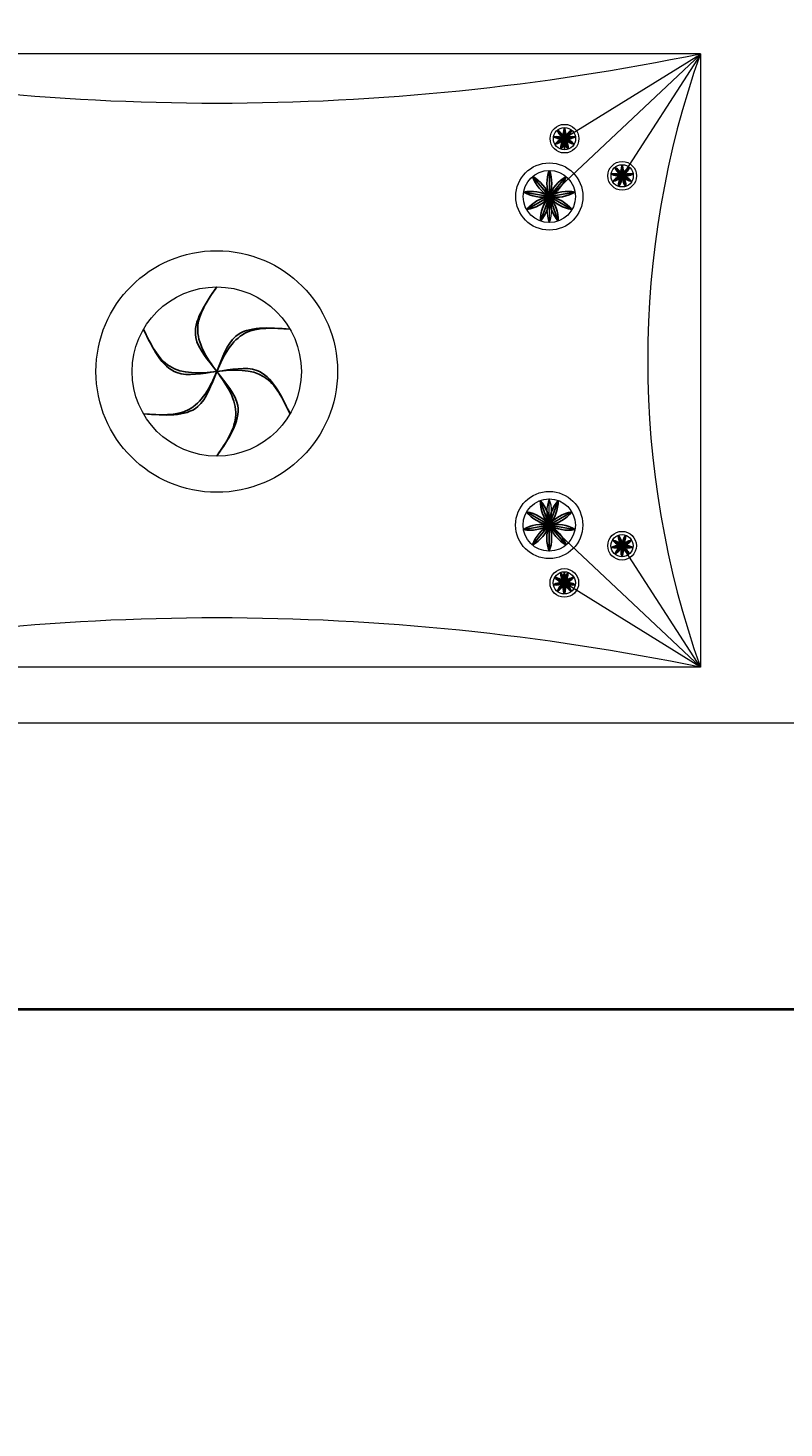
# Model space of a CAD drawing. Units: inches. Extents: x -46 to 1145, y -527 to 760.
# Tile 26 of 57: x 63 to 79, y 222 to 252. Entities that reach past the tile are written whole.
import ezdxf

# ---------------------------------------------------------------- set-up
doc = ezdxf.new("R2010")
doc.units = ezdxf.units.IN
doc.header["$MEASUREMENT"] = 0
for name, color, linetype, lineweight in [('A-ANNO-DIMS', 2, 'Continuous', 18), ('A-FURN', 2, 'Continuous', 13), ('WALLS', 4, 'Continuous', 40)]:
    doc.layers.add(name, color=color, linetype=linetype, lineweight=lineweight)
doc.layers.add('FURNTIURE', color=2, linetype='Continuous')
doc.layers.add('LT', color=9, linetype='Continuous')
doc.styles.get("Standard").update_dxf_attribs({"font": 'arial.ttf'})
doc.dimstyles.get("Standard").update_dxf_attribs({"dimtxt": 0.18, "dimasz": 0.18, "dimexe": 0.18, "dimexo": 0.0625, "dimgap": 0.09, "dimtad": 0, "dimtih": 1, "dimtoh": 1, "dimdec": 0, "dimzin": 0, "dimdsep": 46, "dimlunit": 3, "dimtxsty": 'Standard', "dimcen": 0.09, "dimadec": 0, "dimazin": 0, "dimtfac": 1, "dimtdec": 0, "dimtofl": 0, "dimtmove": 0, "dimatfit": 3, "dimfxl": 1, "dimtolj": 1, "dimtzin": 0, "dimarcsym": 0})

# ---------------------------------------------------------------- blocks, each defined once
blk = doc.blocks.new('*U64')
at = {"layer": 'LT'}
blk.add_line((0, 0.281), (0, -0.281), dxfattribs=at)
for centre, start, end in [((0.734, 0), 159.0676, 200.9324), ((-0.734, 0), 339.0676, 20.9324)]:
    blk.add_arc(centre, 0.786, start, end, dxfattribs=at)
blk = doc.blocks.new('*U65')
at = {"layer": 'LT', "transparency": 16777216}
blk.add_blockref('*U64', (609.936, 444.026), dxfattribs=at)
for p, rotation in [((609.756, 443.96), 40.00000000000002), ((610.117, 443.96), 320), ((609.659, 443.794), 80.00000000000001), ((609.693, 443.605), 120), ((609.84, 443.481), 160), ((610.032, 443.481), 200), ((610.179, 443.605), 240), ((610.213, 443.794), 280)]:
    blk.add_blockref('*U64', p, dxfattribs=dict(at, rotation=rotation))
blk = doc.blocks.new('*U66')
at = {"layer": 'LT'}
blk.add_line((0, 0.12), (0, -0.12), dxfattribs=at)
for centre, start, end in [((0.313, 0), 159.0676, 200.9324), ((-0.313, 0), 339.0676, 20.9324)]:
    blk.add_arc(centre, 0.335, start, end, dxfattribs=at)
blk = doc.blocks.new('*U67')
at = {"layer": 'LT', "transparency": 16777216}
for p, rotation in [((259.495, 188.896), 80.00000000000001), ((259.509, 188.816), 120), ((259.536, 188.967), 40), ((259.572, 188.763), 160), ((259.654, 188.763), 200), ((259.69, 188.967), 320), ((259.716, 188.816), 240), ((259.731, 188.896), 280)]:
    blk.add_blockref('*U66', p, dxfattribs=dict(at, rotation=rotation))
blk.add_blockref('*U66', (259.613, 188.995), dxfattribs=at)
blk = doc.blocks.new('*U68')
at = {"layer": 'LT'}
blk.add_line((0, 0.12), (0, -0.12), dxfattribs=at)
for centre, start, end in [((0.313, 0), 159.0676, 200.9324), ((-0.313, 0), 339.0676, 20.9324)]:
    blk.add_arc(centre, 0.335, start, end, dxfattribs=at)
blk = doc.blocks.new('*U69')
at = {"layer": 'LT', "transparency": 16777216}
for p, rotation in [((259.495, 188.896), 80.00000000000001), ((259.509, 188.816), 120), ((259.536, 188.967), 40), ((259.572, 188.763), 160), ((259.654, 188.763), 200), ((259.69, 188.967), 320), ((259.716, 188.816), 240), ((259.731, 188.896), 280)]:
    blk.add_blockref('*U68', p, dxfattribs=dict(at, rotation=rotation))
blk.add_blockref('*U68', (259.613, 188.995), dxfattribs=at)
blk = doc.blocks.new('*U50')
at = {"layer": 'LT'}
blk.add_line((0, 0.281), (0, -0.281), dxfattribs=at)
for centre, start, end in [((0.734, 0), 159.0676, 200.9324), ((-0.734, 0), 339.0676, 20.9324)]:
    blk.add_arc(centre, 0.786, start, end, dxfattribs=at)
blk = doc.blocks.new('*U51')
at = {"layer": 'LT', "transparency": 16777216}
blk.add_blockref('*U50', (609.936, 444.026), dxfattribs=at)
for p, rotation in [((609.756, 443.96), 40.00000000000002), ((610.117, 443.96), 320), ((609.659, 443.794), 80.00000000000001), ((609.693, 443.605), 120), ((609.84, 443.481), 160), ((610.032, 443.481), 200), ((610.179, 443.605), 240), ((610.213, 443.794), 280)]:
    blk.add_blockref('*U50', p, dxfattribs=dict(at, rotation=rotation))
blk = doc.blocks.new('*U52')
at = {"layer": 'LT'}
blk.add_line((0, 0.12), (0, -0.12), dxfattribs=at)
for centre, start, end in [((0.313, 0), 159.0676, 200.9324), ((-0.313, 0), 339.0676, 20.9324)]:
    blk.add_arc(centre, 0.335, start, end, dxfattribs=at)
blk = doc.blocks.new('*U53')
at = {"layer": 'LT', "transparency": 16777216}
for p, rotation in [((259.495, 188.896), 80.00000000000001), ((259.509, 188.816), 120), ((259.536, 188.967), 40), ((259.572, 188.763), 160), ((259.654, 188.763), 200), ((259.69, 188.967), 320), ((259.716, 188.816), 240), ((259.731, 188.896), 280)]:
    blk.add_blockref('*U52', p, dxfattribs=dict(at, rotation=rotation))
blk.add_blockref('*U52', (259.613, 188.995), dxfattribs=at)
blk = doc.blocks.new('*U54')
at = {"layer": 'LT'}
blk.add_line((0, 0.12), (0, -0.12), dxfattribs=at)
for centre, start, end in [((0.313, 0), 159.0676, 200.9324), ((-0.313, 0), 339.0676, 20.9324)]:
    blk.add_arc(centre, 0.335, start, end, dxfattribs=at)
blk = doc.blocks.new('*U55')
at = {"layer": 'LT', "transparency": 16777216}
for p, rotation in [((259.495, 188.896), 80.00000000000001), ((259.509, 188.816), 120), ((259.536, 188.967), 40), ((259.572, 188.763), 160), ((259.654, 188.763), 200), ((259.69, 188.967), 320), ((259.716, 188.816), 240), ((259.731, 188.896), 280)]:
    blk.add_blockref('*U54', p, dxfattribs=dict(at, rotation=rotation))
blk.add_blockref('*U54', (259.613, 188.995), dxfattribs=at)
blk = doc.blocks.new('*U56')
at = {"layer": 'FURNTIURE'}
blk.add_open_spline([(0.039, 1.82), (-0.218, 1.447), (-0.661, 0.801), (0.102, -0.025), (0.645, -0.928), (0.238, -1.527), (0.039, -1.82)], degree=3, knots=[0, 0, 0, 0, 1.177175, 2.037162, 3.056205, 4.032246, 4.032246, 4.032246, 4.032246], dxfattribs=at)
blk = doc.blocks.new('*U57')
at = {"layer": 'FURNTIURE', "transparency": 16777216}
blk.add_blockref('*U56', (904.302, 663.383), dxfattribs=at)
for p, rotation in [((904.379, 663.383), 180), ((904.321, 663.416), 300), ((904.36, 663.416), 239.9999999999999), ((904.321, 663.349), 59.99999999999999), ((904.36, 663.349), 119.9999999999999)]:
    blk.add_blockref('*U56', p, dxfattribs=dict(at, rotation=rotation))
blk = doc.blocks.new('BED-QUEEN-FURNISHED')
for p, q in [((0, 80), (60, 80)), ((31.2, 78.8), (52, 78.8)), ((31.2, 65.6), (31.2, 78.8)), ((31.2, 78.8), (52, 78.8)), ((31.2, 65.6), (31.2, 78.8)), ((31.2, 78.8), (34.585, 75.613)), ((31.2, 78.8), (32.884, 76.184)), ((31.2, 78.8), (34.126, 76.984)), ((34.126, 76.984), (34.126, 76.745)), ((34.451, 75.739), (34.451, 75.177)), ((34.449, 68.673), (34.449, 69.235)), ((31.195, 65.614), (34.582, 68.799)), ((31.195, 65.614), (32.882, 68.228)), ((34.123, 67.428), (34.123, 67.667)), ((31.195, 65.614), (34.123, 67.428)), ((31.2, 65.6), (52, 65.6)), ((31.2, 65.6), (52, 65.6))]:
    blk.add_line(p, q)
for centre, radius in [((34.126, 76.984), 0.308), ((34.126, 76.984), 0.239), ((32.884, 76.184), 0.308), ((32.884, 76.184), 0.239), ((34.451, 75.739), 0.723), ((34.451, 75.739), 0.562), ((41.604, 72.437), 2.599), ((41.604, 72.437), 1.82), ((34.449, 68.673), 0.723), ((34.449, 68.673), 0.562), ((32.882, 68.228), 0.308), ((32.882, 68.228), 0.239), ((34.123, 67.428), 0.308), ((34.123, 67.428), 0.239)]:
    blk.add_circle(centre, radius)
for centre, radius, start, end in [((41.6, 129.177), 51.439, 258.3356, 281.6644), ((12.546, 72.2), 19.787, 340.5151, 19.4849), ((34.439, 76.865), 0.335, 159.0676, 200.9324), ((33.814, 76.865), 0.335, 339.0676, 20.9324), ((35.185, 75.458), 0.786, 159.0676, 200.9324), ((33.717, 75.458), 0.786, 339.0676, 20.9324), ((35.183, 68.953), 0.786, 159.028, 200.8928), ((33.715, 68.954), 0.786, 339.028, 20.8928), ((34.435, 67.547), 0.335, 159.028, 200.8928), ((33.81, 67.548), 0.335, 339.028, 20.8928), ((41.6, 15.223), 51.439, 78.3356, 101.6644)]:
    blk.add_arc(centre, radius, start, end)
at = {"xscale": -1}
for name, p in [('*U69', (293.739, -111.891)), ('*U67', (292.497, -112.691)), ('*U65', (644.387, -368.006))]:
    blk.add_blockref(name, p, dxfattribs=at)
blk.add_blockref('*U57', (-862.736, -590.946))
at = {"rotation": 179.9603994254766}
for name, p in [('*U51', (644.691, 511.997)), ('*U53', (292.625, 256.925)), ('*U55', (293.866, 256.124))]:
    blk.add_blockref(name, p, dxfattribs=at)
blk = doc.blocks.new('*D685')
at = {"layer": 'A-ANNO-DIMS', "color": 0, "lineweight": -2, "transparency": 16777216}
for p, q in [((183.501, 700.889), (-46.216, 700.889)), ((-46.036, 700.709), (-46.036, 116.385)), ((-46.036, -468.302), (-46.036, 116.021)), ((12.501, -468.482), (-46.216, -468.482))]:
    blk.add_line(p, q, dxfattribs=at)
at = {"layer": 'A-ANNO-DIMS', "color": 0, "transparency": 16777216}
for points in [[(-46.066, 700.709), (-46.006, 700.709), (-46.036, 700.889)], [(-46.066, -468.302), (-46.006, -468.302), (-46.036, -468.482)]]:
    blk.add_solid(points, dxfattribs=at)
at = {"layer": 'Defpoints', "color": 0, "transparency": 16777216}
for p in [(-46.036, 700.889), (183.564, 700.889), (12.564, -468.482)]:
    blk.add_point(p, dxfattribs=at)
at = {"layer": 'A-ANNO-DIMS', "color": 0, "transparency": 16777216, "insert": (-46.036, 116.203), "char_height": 0.18, "attachment_point": 5}
blk.add_mtext('\\A1;1169.4', dxfattribs=at)

msp = doc.modelspace()

# ---------------------------------------------------------------- linework, layer by layer
at = {"layer": 'WALLS'}
msp.add_line((183.5637, 230.5176), (21.5637, 230.5176), dxfattribs=at)

# ---------------------------------------------------------------- block references
at = {"layer": 'A-FURN', "rotation": 180}
msp.add_blockref('BED-QUEEN-FURNISHED', (108.4877, 316.6818), dxfattribs=at)

# ---------------------------------------------------------------- dimensions: what is measured, and where the dimension line sits
at = {"layer": 'A-ANNO-DIMS'}
dim = msp.add_linear_dim(base=(-46.0363, 700.8886), p1=(12.5637, -468.4824), p2=(183.5637, 700.8886), angle=90, dimstyle='Standard', override={"dimdec": 1, "dimlfac": 1, "dimrnd": 0, "dimzin": 0, "dimdsep": 46, "dimlunit": 2}, dxfattribs=at)
dim.commit()
dim.dimension.update_dxf_attribs({"geometry": '*D685', "text_midpoint": (-46.0363, 116.2031)})

doc.saveas('drawing.dxf')
